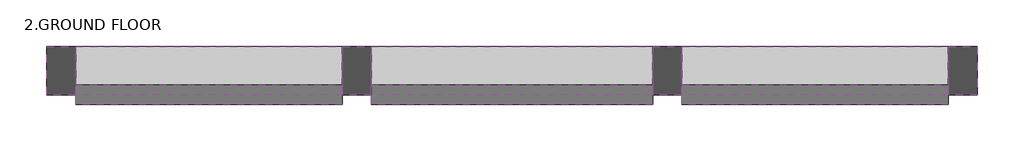
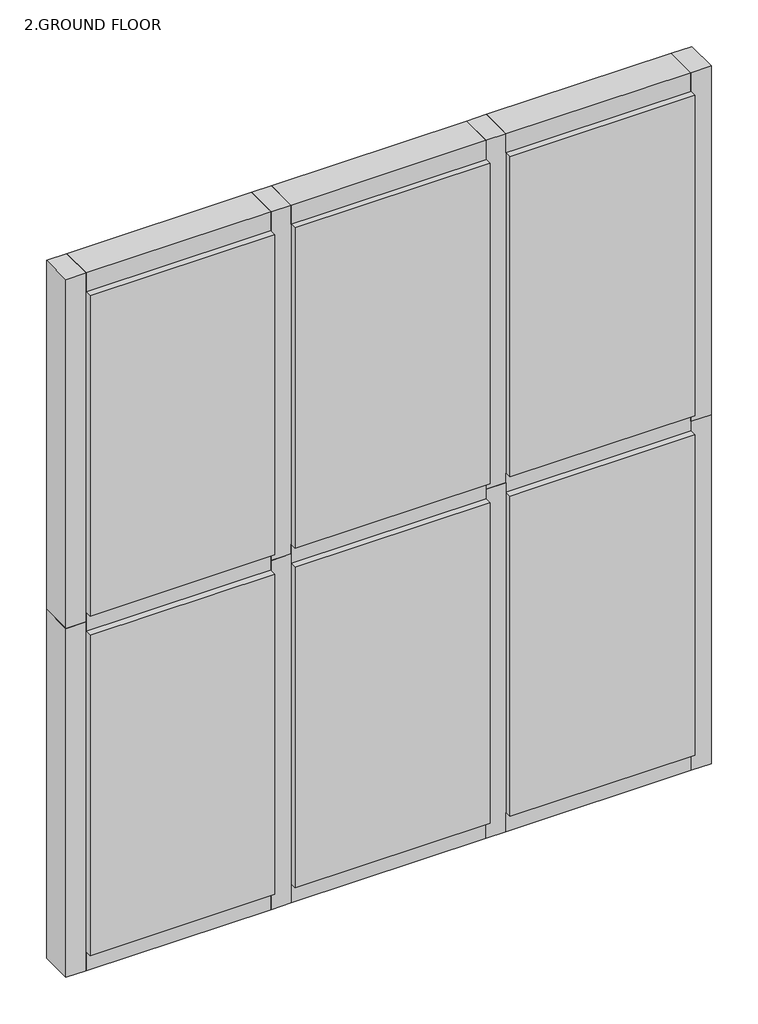
# One storey: 17 members, 6 plates.
"""IFC4 building model written with IfcOpenShell, lengths in millimetres."""

from ifc_helpers import new_model, si_unit, origin, place, context, project, spatial, transform, mapped, element, save
from components import member_07b5019b, member_85007bd8, member_4cd326a7, member_bec67f52, member_bebcb7d7, member_57040902, system_panel_glazed_c3a15102, system_panel_glazed_31ef28de

model = new_model("IFC4")

# Units and contexts
model_context = context("Model", 3, world=origin())
ifc_project = project(units=[si_unit("LENGTHUNIT", "METRE", prefix="MILLI")], contexts=[model_context])

# Site, building, storey
site = spatial("IfcSite", under=ifc_project)
building = spatial("IfcBuilding", under=site)
storey = spatial("IfcBuildingStorey", under=building, Name="2.GROUND FLOOR", Elevation=600.0)

# Members
placement = place(None, origin())
member_shape = member_07b5019b(model_context)
element("IfcMember", 1, ObjectType="Rectangular Mullion : 1.5\" x 2.5\" rectangular", at=placement, inside=storey, context=model_context, shape_type="MappedRepresentation", body=[
    mapped(member_shape, transform((2459.4463749, -5962.873087, 2745.0245486), x_axis=(0.0, 0.0, 1.0), y_axis=(0.0, 1.0, 0.0), z_axis=(-1.0, 0.0, 0.0))),
])
element("IfcMember", 2, ObjectType="Rectangular Mullion : 1.5\" x 2.5\" rectangular", at=placement, inside=storey, context=model_context, shape_type="MappedRepresentation", body=[
    mapped(member_shape, transform((3253.1963749, -5962.873087, 2745.0245486), x_axis=(0.0, 0.0, 1.0), y_axis=(0.0, 1.0, 0.0), z_axis=(-1.0, 0.0, 0.0))),
])
element("IfcMember", 3, ObjectType="Rectangular Mullion : 1.5\" x 2.5\" rectangular", at=placement, inside=storey, context=model_context, shape_type="MappedRepresentation", body=[
    mapped(member_shape, transform((3602.4463749, -5962.873087, 1351.6312076), x_axis=(0.0, 0.0, -1.0), y_axis=(0.0, 1.0, 0.0), z_axis=(1.0, 0.0, 0.0))),
])
element("IfcMember", 4, ObjectType="Rectangular Mullion : 1.5\" x 2.5\" rectangular", at=placement, inside=storey, context=model_context, shape_type="MappedRepresentation", body=[
    mapped(member_shape, transform((2808.6963749, -5962.873087, 1351.6312076), x_axis=(0.0, 0.0, -1.0), y_axis=(0.0, 1.0, 0.0), z_axis=(1.0, 0.0, 0.0))),
])
member_2_shape = member_85007bd8(model_context)
element("IfcMember", 5, ObjectType="Rectangular Mullion : 1.5\" x 2.5\" rectangular", at=placement, inside=storey, context=model_context, shape_type="MappedRepresentation", body=[
    mapped(member_2_shape, transform((2827.7463749, -5962.873087, 1351.6312076), x_axis=(-1.0, 0.0, 0.0), y_axis=(0.0, 1.0, 0.0), z_axis=(0.0, 0.0, -1.0))),
])
element("IfcMember", 6, ObjectType="Rectangular Mullion : 1.5\" x 2.5\" rectangular", at=placement, inside=storey, context=model_context, shape_type="MappedRepresentation", body=[
    mapped(member_2_shape, transform((3234.1463749, -5962.873087, 1351.6312076), x_axis=(-1.0, 0.0, 0.0), y_axis=(0.0, 1.0, 0.0), z_axis=(0.0, 0.0, -1.0))),
])
member_3_shape = member_4cd326a7(model_context)
element("IfcMember", 7, ObjectType="Rectangular Mullion : 1.5\" x 2.5\" rectangular", at=placement, inside=storey, context=model_context, shape_type="MappedRepresentation", body=[
    mapped(member_3_shape, transform((3253.1963749, -5962.873087, 2048.3278781), x_axis=(0.0, 0.0, 1.0), y_axis=(0.0, 1.0, 0.0), z_axis=(-1.0, 0.0, 0.0))),
])
element("IfcMember", 8, ObjectType="Rectangular Mullion : 1.5\" x 2.5\" rectangular", at=placement, inside=storey, context=model_context, shape_type="MappedRepresentation", body=[
    mapped(member_3_shape, transform((2459.4463749, -5962.873087, 2048.3278781), x_axis=(0.0, 0.0, 1.0), y_axis=(0.0, 1.0, 0.0), z_axis=(-1.0, 0.0, 0.0))),
])
member_4_shape = member_bec67f52(model_context)
element("IfcMember", 9, ObjectType="Rectangular Mullion : 1.5\" x 2.5\" rectangular", at=placement, inside=storey, context=model_context, shape_type="MappedRepresentation", body=[
    mapped(member_4_shape, transform((2846.7963749, -5962.873087, 2048.3278781), x_axis=(0.0, 0.0, 1.0), y_axis=(0.0, 1.0, 0.0), z_axis=(-1.0, 0.0, 0.0))),
])
member_5_shape = member_bebcb7d7(model_context)
element("IfcMember", 10, ObjectType="Rectangular Mullion : 1.5\" x 2.5\" rectangular", at=placement, inside=storey, context=model_context, shape_type="MappedRepresentation", body=[
    mapped(member_5_shape, transform((3215.0963749, -5962.873087, 1351.6312076), x_axis=(0.0, 0.0, -1.0), y_axis=(0.0, 1.0, 0.0), z_axis=(1.0, 0.0, 0.0))),
])
element("IfcMember", 11, ObjectType="Rectangular Mullion : 1.5\" x 2.5\" rectangular", at=placement, inside=storey, context=model_context, shape_type="MappedRepresentation", body=[
    mapped(member_5_shape, transform((2846.7963749, -5962.873087, 2745.0245486), x_axis=(0.0, 0.0, 1.0), y_axis=(0.0, 1.0, 0.0), z_axis=(-1.0, 0.0, 0.0))),
])
element("IfcMember", 12, ObjectType="Rectangular Mullion : 1.5\" x 2.5\" rectangular", at=placement, inside=storey, context=model_context, shape_type="MappedRepresentation", body=[
    mapped(member_2_shape, transform((2827.7463749, -5962.873087, 2048.3278781), x_axis=(-1.0, 0.0, 0.0), y_axis=(0.0, 1.0, 0.0), z_axis=(0.0, 0.0, -1.0))),
])
element("IfcMember", 13, ObjectType="Rectangular Mullion : 1.5\" x 2.5\" rectangular", at=placement, inside=storey, context=model_context, shape_type="MappedRepresentation", body=[
    mapped(member_2_shape, transform((3234.1463749, -5962.873087, 2048.3278781), x_axis=(-1.0, 0.0, 0.0), y_axis=(0.0, 1.0, 0.0), z_axis=(0.0, 0.0, -1.0))),
])
member_6_shape = member_57040902(model_context)
element("IfcMember", 14, ObjectType="Rectangular Mullion : 1.5\" x 2.5\" rectangular", at=placement, inside=storey, context=model_context, shape_type="MappedRepresentation", body=[
    mapped(member_6_shape, transform((3640.5463749, -5962.873087, 2745.0245486), x_axis=(1.0, 0.0, 0.0), y_axis=(0.0, 1.0, 0.0), z_axis=(0.0, 0.0, 1.0))),
])
element("IfcMember", 15, ObjectType="Rectangular Mullion : 1.5\" x 2.5\" rectangular", at=placement, inside=storey, context=model_context, shape_type="MappedRepresentation", body=[
    mapped(member_6_shape, transform((2421.3463749, -5962.873087, 1351.6312076), x_axis=(-1.0, 0.0, 0.0), y_axis=(0.0, 1.0, 0.0), z_axis=(0.0, 0.0, -1.0))),
])
element("IfcMember", 16, ObjectType="Rectangular Mullion : 1.5\" x 2.5\" rectangular", at=placement, inside=storey, context=model_context, shape_type="MappedRepresentation", body=[
    mapped(member_6_shape, transform((2421.3463749, -5962.873087, 2048.3278781), x_axis=(-1.0, 0.0, 0.0), y_axis=(0.0, 1.0, 0.0), z_axis=(0.0, 0.0, -1.0))),
])
element("IfcMember", 17, ObjectType="Rectangular Mullion : 1.5\" x 2.5\" rectangular", at=placement, inside=storey, context=model_context, shape_type="MappedRepresentation", body=[
    mapped(member_6_shape, transform((3640.5463749, -5962.873087, 2048.3278781), x_axis=(1.0, 0.0, 0.0), y_axis=(0.0, 1.0, 0.0), z_axis=(0.0, 0.0, 1.0))),
])

# Plates
system_panel_glazed_shape = system_panel_glazed_c3a15102(model_context)
element("IfcPlate", 18, ObjectType="System Panel : Glazed", at=placement, inside=storey, context=model_context, shape_type="MappedRepresentation", body=[
    mapped(system_panel_glazed_shape, transform((3427.8213749, -5962.873087, 1389.7312076), x_axis=(-1.0, 0.0, 0.0), y_axis=(0.0, -1.0, 0.0), z_axis=(0.0, 0.0, 1.0))),
])
element("IfcPlate", 19, ObjectType="System Panel : Glazed", at=placement, inside=storey, context=model_context, shape_type="MappedRepresentation", body=[
    mapped(system_panel_glazed_shape, transform((2634.0713749, -5962.873087, 1389.7312076), x_axis=(-1.0, 0.0, 0.0), y_axis=(0.0, -1.0, 0.0), z_axis=(0.0, 0.0, 1.0))),
])
element("IfcPlate", 20, ObjectType="System Panel : Glazed", at=placement, inside=storey, context=model_context, shape_type="MappedRepresentation", body=[
    mapped(system_panel_glazed_shape, transform((3427.8213749, -5962.873087, 2067.3778781), x_axis=(-1.0, 0.0, 0.0), y_axis=(0.0, -1.0, 0.0), z_axis=(0.0, 0.0, 1.0))),
])
element("IfcPlate", 21, ObjectType="System Panel : Glazed", at=placement, inside=storey, context=model_context, shape_type="MappedRepresentation", body=[
    mapped(system_panel_glazed_shape, transform((2634.0713749, -5962.873087, 2067.3778781), x_axis=(-1.0, 0.0, 0.0), y_axis=(0.0, -1.0, 0.0), z_axis=(0.0, 0.0, 1.0))),
])
system_panel_glazed_2_shape = system_panel_glazed_31ef28de(model_context)
element("IfcPlate", 22, ObjectType="System Panel : Glazed", at=placement, inside=storey, context=model_context, shape_type="MappedRepresentation", body=[
    mapped(system_panel_glazed_2_shape, transform((3030.9463749, -5962.873087, 1389.7312076), x_axis=(-1.0, 0.0, 0.0), y_axis=(0.0, -1.0, 0.0), z_axis=(0.0, 0.0, 1.0))),
])
element("IfcPlate", 23, ObjectType="System Panel : Glazed", at=placement, inside=storey, context=model_context, shape_type="MappedRepresentation", body=[
    mapped(system_panel_glazed_2_shape, transform((3030.9463749, -5962.873087, 2067.3778781), x_axis=(-1.0, 0.0, 0.0), y_axis=(0.0, -1.0, 0.0), z_axis=(0.0, 0.0, 1.0))),
])

save(model, "model.ifc")

# Revit data of these elements
# Type "Rectangular Mullion : 1.5\" x 2.5\" rectangular"
#   built-in parameter 1007304 = 0.208333 (stored number, unit not read)
#   built-in parameter 1007301 = 0.0625 (stored number, unit not read)
#   built-in parameter 1007300 = 0.0625 (stored number, unit not read)
# Type "System Panel : Glazed"
#   Construction Type Id = "GSP4R"
#   Analytic Construction = "1/8 in Pilkington single glazing"
#   Visual Light Transmittance = 0.9
#   Solar Heat Gain Coefficient = 0.86
#   Heat Transfer Coefficient (U) = 1.18115 BTU/(h·ft²·°F)
#   Define Thermal Properties by = 1
# Elements 1, 2, 3, 4, 5, 6, 7, 8, 9, 10, 11, 12, 13, 14, 15, 16, 17 (IfcMember, "Rectangular Mullion : 1.5\" x 2.5\" rectangular")
#   Phase Created = New Construction
#   Materials on its faces: "Damp-proofing"
# Elements 18, 19, 20, 21, 22, 23 (IfcPlate, "System Panel : Glazed")
#   Phase Created = New Construction
#   Materials on its faces: "Glass"
# Materials
#   "Damp-proofing": class "Generic", colour RGB 127 127 127, transparency 0, Description = "Damp-proofing", Cost = 0
#   "Glass": class "Glass", colour RGB 0 128 192, transparency 0.75, Description = "Soda Lime Glass", Cost = 0
